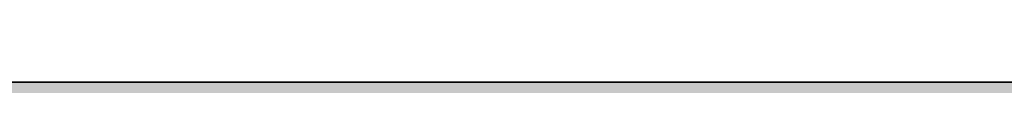
# Model space of a CAD drawing. Units: inches. Extents: x 2091 to 2899, y 967 to 2217.
# Tile 87 of 256: x 2251.287593 to 2251.296488, y 1099.919027 to 1099.919418. Entities that reach past the tile are written whole.
import ezdxf

# ---------------------------------------------------------------- set-up
doc = ezdxf.new("R2010")
doc.units = ezdxf.units.IN
doc.layers.add('A-WALL-PATT', color=141, linetype='Continuous', lineweight=13, true_color=0xadddf7)
doc.layers.add('L-SITE-WALL', color=7, linetype='Continuous', lineweight=35)

msp = doc.modelspace()

# ---------------------------------------------------------------- hatches: boundary and pattern name
at = {"layer": 'A-WALL-PATT'}
h = msp.add_hatch(color=256, dxfattribs=at)
h.dxf.hatch_style = 1
h.paths.add_polyline_path([(2212.1436027, 1941.4190588), (2387.6436027, 1941.4190588), (2387.6436027, 1824.4190588), (2392.1436027, 1824.4190588), (2392.1436027, 1941.4190588), (2609.6436027, 1941.4190588), (2609.6436027, 1825.9190588), (2614.1436027, 1825.9190588), (2614.1436027, 1941.4190588), (2794.1436027, 1941.4190588), (2794.1436027, 1928.7621663), (2803.1436027, 1928.7621663), (2803.1436027, 2050.9190588), (2203.1436027, 2050.9190588), (2203.1436027, 1900.7578592), (2212.1436027, 1900.7578592)])
h.paths.add_polyline_path([(2212.1436027, 1945.9190588), (2212.1436027, 2041.9190588), (2794.1436027, 2041.9190588), (2794.1436027, 1945.9190588), (2402.2482445, 1945.9190588), (2401.1024337, 1945.7758325), (2398.7024337, 1945.7758325)], flags=16)
h.paths.add_polyline_path([(2230.2298609, 1948.0627926), (2227.3498609, 1949.5027926), (2225.9098609, 1951.9027926), (2223.9898609, 1952.8627926), (2223.0298609, 1955.2627926), (2222.0698609, 1959.5827926), (2222.0698609, 1963.4227926), (2223.0298609, 1965.6627926), (2223.9898609, 1965.3427926), (2225.58591, 1963.860747), (2226.9115333, 1964.9572589), (2226.9488609, 1965.9387926), (2227.7783187, 1966.9521426), (2228.1999161, 1968.8787044), (2230.7098609, 1964.8627926), (2233.5898609, 1966.3027926), (2233.607309, 1966.3318728), (2233.7726595, 1964.9382048), (2234.6338015, 1963.6764729), (2235.0298609, 1963.9027926), (2236.2820348, 1965.5723578), (2235.9898609, 1962.9427926), (2237.9545121, 1957.5400019), (2238.3898609, 1957.9027926), (2239.2158609, 1960.3057926), (2238.6545655, 1966.3849599), (2238.6927918, 1966.4380694), (2238.8405779, 1967.4997069), (2238.7802908, 1967.6874864), (2238.8805378, 1967.7867629), (2238.6668609, 1966.2517926), (2239.2158609, 1960.3057926), (2238.3898609, 1957.9027926), (2236.9498609, 1956.7027926), (2234.5498609, 1949.9827926)], flags=0)
h.paths.add_polyline_path([(2278.0119735, 1948.0627926), (2276.4964266, 1947.8733492), (2275.8498328, 1947.6886081), (2274.6519735, 1947.1027926)], flags=0)
h.paths.add_polyline_path([(2269.8519735, 1955.7427926), (2268.2761762, 1956.6293287), (2270.8673022, 1956.3483982), (2269.3719735, 1958.1427926), (2268.7149641, 1959.1923253), (2270.5698328, 1958.7286081), (2268.5807252, 1961.9060872), (2270.8119735, 1960.8918835), (2270.8119735, 1963.4227926), (2271.3933148, 1964.7792556), (2270.2917623, 1966.1561963), (2271.7719735, 1965.6627926), (2272.1413868, 1966.5247568), (2273.9298328, 1965.9286081), (2275.6303855, 1968.054299), (2276.331938, 1966.72186), (2276.5204313, 1966.9521426), (2276.9420286, 1968.8787044), (2277.7342926, 1967.6110821), (2278.1398879, 1969.4645199), (2279.6591239, 1967.0337425), (2280.4119735, 1966.7827926), (2280.9493019, 1967.5887851), (2281.6098328, 1967.3686081), (2282.1332658, 1968.1537576), (2282.3492351, 1966.3334449), (2282.3498491, 1966.3325853), (2283.40755, 1968.0954201), (2283.7126314, 1965.5240203), (2284.3202211, 1964.6337894), (2284.5118085, 1964.8892393), (2284.2349735, 1965.7047926), (2284.500472, 1967.3189584), (2284.9079444, 1965.4174205), (2285.3963134, 1966.0685791), (2285.4328328, 1966.2906081), (2285.4733384, 1966.1712791), (2286.3539194, 1967.345387), (2286.2220067, 1966.1581734), (2287.6634921, 1968.0801538), (2287.7139735, 1968.4427926), (2288.4815994, 1969.0166793), (2288.5739928, 1968.7288966), (2288.9174612, 1969.0690403), (2288.6068328, 1966.8376081), (2288.9287261, 1963.3513103), (2288.9349735, 1963.3567926), (2288.9297314, 1963.3404224), (2289.015281, 1962.4138692), (2290.1112234, 1963.8751258), (2290.1328328, 1963.9426081), (2290.2176723, 1964.0170576), (2290.1112234, 1963.8751258), (2289.1558328, 1960.8916081), (2288.5940356, 1959.2572271), (2288.5719735, 1959.1027926), (2289.5319735, 1960.5427926), (2290.0119735, 1962.4627926), (2290.1918401, 1962.6426592), (2289.7698328, 1959.6886081), (2286.8898328, 1957.2886081), (2284.4898328, 1950.5686081), (2283.3146576, 1950.046308), (2283.2919735, 1949.9827926), (2280.2900585, 1948.6486081), (2281.1298328, 1948.6486081), (2282.5698328, 1948.1686081), (2283.2047262, 1948.0627926), (2278.9719735, 1948.0627926), (2276.0919735, 1949.5027926), (2274.6519735, 1951.9027926), (2272.7319735, 1952.8627926)], flags=0)
h.paths.add_polyline_path([(2271.1588684, 1958.0217654), (2272.9698328, 1955.8486081), (2272.0098328, 1960.1686081), (2272.0098328, 1964.0086081), (2272.6244258, 1965.4426583), (2274.3280226, 1963.860747), (2275.6536458, 1964.9572589), (2275.6377429, 1964.5390903), (2277.4122311, 1966.0068885), (2277.0329735, 1965.1567926), (2276.829924, 1964.9755966), (2276.7660116, 1963.2950136), (2277.4496351, 1962.6602203), (2279.4519735, 1964.8627926), (2282.3319735, 1966.3027926), (2283.5298328, 1966.8886081), (2283.2945117, 1966.7709476), (2283.9129934, 1963.8846999), (2284.8992493, 1964.4482747), (2284.7319735, 1962.9427926), (2286.6966247, 1957.5400019), (2287.1319735, 1957.9027926), (2287.5419128, 1959.0953883), (2287.7793955, 1958.4423109), (2285.6827383, 1956.6950966), (2285.8765033, 1959.7953357), (2284.7319735, 1962.9427926), (2284.8992493, 1964.4482747), (2283.9129934, 1963.8846999), (2284.2238328, 1962.4341157), (2283.4243649, 1963.6054836), (2281.6098328, 1962.5686081), (2281.1298328, 1960.1686081), (2282.0898328, 1956.3286081), (2283.0498328, 1952.9686081), (2282.5698328, 1950.5686081), (2280.1698328, 1948.6486081), (2279.883316, 1948.7918666), (2278.9719735, 1948.0627926), (2278.9719735, 1949.0227926), (2278.6723132, 1949.3973679), (2277.2898328, 1950.0886081), (2275.8498328, 1952.4886081), (2273.9298328, 1953.4486081), (2272.4898328, 1954.8886081), (2271.9216473, 1954.8886081), (2271.7719735, 1955.2627926)], flags=0)
h.paths.add_polyline_path([(2311.994146, 1955.7427926), (2312.0627174, 1955.6742211), (2312.0550999, 1955.7085002)], flags=0)
h.paths.add_polyline_path([(2331.956146, 1963.9517926), (2333.396146, 1965.3917926), (2331.077146, 1963.3567926), (2330.998603, 1963.1115166)], flags=0)
h.paths.add_polyline_path([(2310.554146, 1954.3027926), (2307.0398066, 1956.2799434), (2310.7629029, 1955.8762843), (2312.474146, 1953.8227926), (2313.434146, 1951.4227926), (2315.354146, 1950.4627926), (2316.794146, 1948.0627926), (2317.466146, 1947.7267926), (2319.3686915, 1947.9646108), (2317.754146, 1949.9827926), (2317.5695306, 1950.6104849), (2316.794146, 1951.9027926), (2314.874146, 1952.8627926), (2313.914146, 1955.2627926), (2311.514146, 1958.1427926), (2309.3754889, 1961.5591681), (2311.514146, 1960.3370783), (2311.514146, 1961.9827926), (2310.6046723, 1963.1196347), (2311.726605, 1962.4785303), (2312.4183321, 1964.09256), (2312.2559642, 1964.2955198), (2313.194146, 1963.9827926), (2313.914146, 1965.6627926), (2314.6467776, 1965.418582), (2315.354146, 1966.3027926), (2316.794146, 1967.7427926), (2316.1574354, 1966.9469043), (2317.0341105, 1965.28186), (2317.2226038, 1965.5121426), (2317.7770481, 1968.0457711), (2318.4741105, 1966.72186), (2318.6626038, 1966.9521426), (2319.0842012, 1968.8787044), (2321.2070492, 1965.4821474), (2322.1614187, 1966.9137017), (2322.554146, 1966.7827926), (2322.7859877, 1967.1305552), (2322.881646, 1966.3242926), (2323.3120408, 1965.7217399), (2323.6512889, 1965.891364), (2324.3964998, 1967.1333822), (2324.6569446, 1964.9382048), (2324.971986, 1964.476611), (2325.3872804, 1967.001499), (2325.9408127, 1964.4183481), (2327.2289286, 1966.1358361), (2327.1663199, 1965.5723578), (2328.0591386, 1966.7627827), (2328.2245759, 1966.2474864), (2329.6679714, 1967.6769101), (2329.6645759, 1967.6874864), (2329.7648229, 1967.7867629), (2329.551146, 1966.2517926), (2330.100146, 1960.3057926), (2329.3328143, 1958.0734703), (2329.3130649, 1957.935225), (2329.634146, 1958.2027926), (2330.234146, 1959.1027926), (2330.714146, 1961.0227926), (2331.034146, 1961.3427926), (2330.714146, 1959.1027926), (2329.634146, 1958.2027926), (2329.274146, 1957.6627926), (2327.7121121, 1956.3610977), (2325.434146, 1949.9827926), (2324.3337687, 1949.493736), (2323.994146, 1948.5427926), (2319.674146, 1946.6227926), (2316.794146, 1948.0627926), (2315.354146, 1950.4627926), (2313.434146, 1951.4227926)], flags=0)
h.paths.add_polyline_path([(2321.3356845, 1947.9520233), (2321.114146, 1948.0627926), (2321.114146, 1949.0227926), (2319.194146, 1951.4227926), (2316.794146, 1959.5827926), (2316.6632369, 1959.5827926), (2315.354146, 1958.1427926), (2314.394146, 1958.1427926), (2313.1483033, 1958.7090847), (2312.954146, 1959.5827926), (2312.954146, 1960.8918835), (2315.834146, 1959.5827926), (2316.6632369, 1959.5827926), (2317.3147094, 1960.2994123), (2315.0301951, 1962.420747), (2316.3558184, 1963.5172589), (2316.3723369, 1963.9516153), (2316.4701951, 1963.860747), (2317.7958184, 1964.9572589), (2317.7552187, 1963.8896871), (2319.175146, 1965.1567926), (2319.4984065, 1965.8813724), (2321.114146, 1965.3427926), (2323.2358851, 1962.3723578), (2325.6863494, 1963.7726231), (2325.5427886, 1962.4805756), (2325.1987827, 1963.4940135), (2324.4785097, 1963.0824289), (2324.9260053, 1960.9941157), (2324.0780866, 1962.2364729), (2322.4147912, 1961.2860184), (2322.074146, 1959.5827926), (2323.034146, 1955.7427926), (2323.994146, 1952.3827926), (2323.514146, 1949.9827926), (2322.1427174, 1948.8856497), (2322.074146, 1948.5427926)], flags=0)
h.paths.add_polyline_path([(2320.2074794, 1963.3374592), (2320.154146, 1963.4227926), (2320.394146, 1963.5427926)], flags=0)
h.paths.add_polyline_path([(2353.8505274, 1965.8105004), (2354.0305274, 1965.7505004), (2354.3305274, 1966.4505004), (2354.3305274, 1966.9305004)], flags=0)
h.paths.add_polyline_path([(2359.0205825, 1969.0264122), (2359.0983824, 1968.9019323), (2359.2335274, 1969.5195004), (2359.2335274, 1969.9995004)], flags=0)
h.paths.add_polyline_path([(2358.2566937, 1966.6816724), (2357.983601, 1966.3480346), (2358.211267, 1966.1461745), (2358.4104918, 1966.3895678)], flags=0)
h.paths.add_polyline_path([(2357.7684731, 1966.0587777), (2357.7321997, 1965.1049667), (2357.751047, 1965.1205565), (2357.7695274, 1965.6065004), (2357.7695274, 1966.057843)], flags=0)
h.paths.add_polyline_path([(2359.1115274, 1965.3045004), (2359.1115274, 1964.8245004), (2359.8445274, 1966.4675004), (2359.8445274, 1966.9475004)], flags=0)
h.paths.add_polyline_path([(2360.2236843, 1966.6214493), (2360.6985274, 1969.3625004), (2360.6985274, 1969.8425004), (2360.2105274, 1967.0255004), (2360.2105274, 1966.6425004)], flags=0)
h.paths.add_polyline_path([(2363.4505274, 1967.8905004), (2363.4505274, 1968.3705004), (2362.4905274, 1966.9305004), (2362.6560446, 1966.6987763)], flags=0)
h.paths.add_polyline_path([(2364.4755226, 1966.0788259), (2365.8505274, 1968.3705004), (2365.8505274, 1968.8505004), (2364.4279755, 1966.4795806)], flags=0)
h.paths.add_polyline_path([(2366.3135274, 1965.8525004), (2366.3667086, 1965.6958291), (2366.8025274, 1968.3455004), (2366.8025274, 1968.8255004)], flags=0)
h.paths.add_polyline_path([(2367.16531, 1965.8035439), (2367.2905274, 1966.9305004), (2367.2905274, 1967.4105004), (2367.1027013, 1965.7200656)], flags=0)
h.paths.add_polyline_path([(2370.0365274, 1959.9735004), (2371.0135274, 1963.0245004), (2371.0135274, 1963.5045004), (2370.0365274, 1960.4535004)], flags=0)
h.paths.add_polyline_path([(2371.6105274, 1960.2105004), (2372.5705274, 1961.6505004), (2372.5705274, 1962.1305004), (2371.8025274, 1960.9785004)], flags=0)
h.paths.add_polyline_path([(2350.8736661, 1956.0050856), (2351.9305274, 1955.8905004), (2354.4905274, 1953.3305004), (2353.8505274, 1954.9305004), (2351.4505274, 1957.8105004), (2347.9355274, 1963.4255004), (2347.9355274, 1963.9055004), (2351.4505274, 1958.2905004), (2353.7050728, 1955.5850458), (2352.8905274, 1959.2505004), (2352.8905274, 1959.7305004), (2352.8905274, 1961.9247861), (2356.7305274, 1959.7305004), (2358.454471, 1961.6268384), (2354.8105274, 1965.0105004), (2355.0308552, 1965.2859102), (2358.6910907, 1961.8871201), (2361.5305274, 1965.0105004), (2364.3764954, 1966.4334844), (2364.5243939, 1965.1869106), (2365.454468, 1963.8241807), (2365.8810728, 1964.0679549), (2365.3705274, 1966.4505004), (2365.3705274, 1966.9305004), (2366.8105274, 1960.2105004), (2366.8105274, 1959.7305004), (2366.3887092, 1952.9814095), (2367.7705274, 1956.8505004), (2368.641225, 1957.5760818), (2366.8105274, 1962.6105004), (2366.8105274, 1963.0905004), (2368.7751785, 1957.6877097), (2369.2105274, 1958.0505004), (2370.0015924, 1960.3518674), (2369.4752319, 1966.0526677), (2369.5134582, 1966.1057772), (2369.514173, 1966.1109121), (2369.4752319, 1966.5326677), (2369.5134582, 1966.5857772), (2369.614635, 1967.3125914), (2369.1825274, 1968.6585004), (2369.1825274, 1969.1385004), (2369.6009573, 1967.8351942), (2369.7012042, 1967.9344708), (2369.7179468, 1968.054743), (2370.1451758, 1968.3741448), (2369.7787075, 1968.0112238), (2369.7012042, 1967.4544708), (2370.4681613, 1968.2140038), (2369.674936, 1967.2657706), (2369.514173, 1966.1109121), (2370.0365274, 1960.4535004), (2370.0365274, 1959.9735004), (2369.441756, 1958.2431909), (2370.6505274, 1959.2505004), (2371.0458215, 1962.0175592), (2371.1305274, 1962.1305004), (2370.6505274, 1958.7705004), (2367.7705274, 1956.3705004), (2365.3705274, 1949.6505004), (2362.0790988, 1948.1876432), (2363.4505274, 1947.7305004), (2361.0505274, 1947.7305004), (2360.0905274, 1947.7305004), (2357.1038607, 1947.3571671), (2360.0905274, 1948.2105004), (2358.1705274, 1949.1705004), (2356.7305274, 1951.5705004), (2354.8105274, 1952.5305004), (2351.9305274, 1955.4105004)], flags=0)
h.paths.add_polyline_path([(2361.0505274, 1948.6905004), (2359.1305274, 1951.0905004), (2356.7305274, 1959.2505004), (2355.7705274, 1959.2505004), (2352.8905274, 1960.5595913), (2352.8905274, 1961.4447861), (2355.8905274, 1959.7305004), (2356.7305274, 1959.7305004), (2356.837194, 1959.3678337), (2361.5305274, 1964.5305004), (2363.2484221, 1965.3894478), (2364.92531, 1963.0418047), (2362.4905274, 1961.6505004), (2362.0638607, 1959.5171671), (2362.9705274, 1955.8905004), (2363.9305274, 1952.5305004), (2363.9305274, 1952.0505004), (2363.4505274, 1949.6505004), (2361.0505274, 1947.7305004)], flags=0)
h.paths.add_polyline_path([(2359.1305274, 1951.5705004), (2359.2905274, 1951.3705004), (2361.0505274, 1954.4505004), (2361.0505274, 1954.9305004)], flags=0)
h.paths.add_polyline_path([(2357.2195274, 1966.5455004), (2356.7925274, 1968.8145004), (2356.7925274, 1969.2945004), (2357.2195274, 1967.0255004)], flags=0)
h.paths.add_polyline_path([(2361.0505274, 1954.4505004), (2361.5305274, 1958.7705004), (2361.5305274, 1959.2505004), (2361.0505274, 1954.9305004)], flags=0)
h.paths.add_polyline_path([(2402.5482874, 1948.4860764), (2402.3024337, 1948.4158325), (2402.5904337, 1948.4158325)], flags=0)
h.paths.add_polyline_path([(2394.1424337, 1956.0958325), (2395.6850518, 1954.5532144), (2396.7204952, 1953.9706788), (2396.0624337, 1955.6158325), (2395.2413811, 1956.6010956), (2395.8789043, 1956.4417148), (2395.1024337, 1959.9358325), (2395.1024337, 1963.7758325), (2396.0624337, 1966.0158325), (2397.0224337, 1965.6958325), (2398.6184828, 1964.2137869), (2399.9441061, 1965.3102988), (2399.9814337, 1966.2918325), (2400.8108915, 1967.3051825), (2401.2324888, 1969.2317443), (2403.5379492, 1965.5430077), (2403.9419843, 1967.3893156), (2404.7024337, 1967.1358325), (2405.4603284, 1966.0747799), (2406.6224337, 1966.6558325), (2406.6398818, 1966.6849127), (2406.8052323, 1965.2912447), (2406.9256943, 1965.1147456), (2407.3424337, 1964.9758325), (2407.8743256, 1965.7736703), (2408.1691004, 1964.3980547), (2409.3146076, 1965.9253977), (2409.2174583, 1965.0510538), (2409.4452323, 1963.1312447), (2410.3063743, 1961.8695128), (2410.7024337, 1962.0958325), (2411.4422687, 1963.0822792), (2411.1654337, 1963.8978325), (2411.6164263, 1966.6397566), (2411.7253645, 1966.7911093), (2411.8731507, 1967.8527468), (2411.8128636, 1968.0405263), (2411.9131106, 1968.1398028), (2411.6994337, 1966.6048325), (2412.2484337, 1960.6588325), (2413.2254337, 1963.7098325), (2414.3779002, 1964.7211603), (2414.5131507, 1965.6927468), (2414.4528636, 1965.8805263), (2414.5531106, 1965.9798028), (2414.3779002, 1964.7211603), (2414.5198172, 1964.8456973), (2414.3653645, 1964.6311093), (2414.3394337, 1964.4448325), (2414.8884337, 1958.4988325), (2414.0624337, 1956.0958325), (2412.6224337, 1954.8958325), (2410.1713699, 1948.0328538), (2410.0167194, 1948.0844039), (2405.9024337, 1946.2558325), (2405.9024337, 1947.2158325), (2405.2042519, 1948.0885598), (2404.2224337, 1948.4158325), (2403.2624337, 1948.4158325), (2400.3824337, 1949.8558325), (2399.6624337, 1951.0558325), (2397.9824337, 1952.7358325), (2397.0224337, 1953.2158325), (2395.6850518, 1954.5532144), (2392.6567764, 1956.2569078)], flags=0)
h.paths.add_polyline_path([(2409.0856501, 1964.4074407), (2409.1303635, 1964.2757154), (2409.2624337, 1964.4958325)], flags=0)
h.paths.add_polyline_path([(2397.7424337, 1961.6158325), (2398.7024337, 1963.8558325), (2399.6624337, 1963.5358325), (2401.4265631, 1965.7409942), (2401.7914151, 1966.5588003), (2402.0714337, 1965.0708325), (2402.8355074, 1964.3933667), (2403.2623982, 1964.9148999), (2403.3381187, 1964.771086), (2402.6155159, 1963.9762229), (2402.4986125, 1960.9022379), (2403.5429971, 1959.9324522), (2404.4132029, 1960.8896786), (2404.7024337, 1962.3358325), (2407.9163468, 1964.1723542), (2409.5202115, 1961.9269436), (2410.9870849, 1957.8930418), (2411.4224337, 1958.2558325), (2412.0479637, 1960.075625), (2412.4103407, 1959.0790883), (2411.6756205, 1958.4668215), (2411.6624337, 1958.2558325), (2411.6260701, 1958.4255295), (2409.9824337, 1957.0558325), (2407.5824337, 1950.3358325), (2403.2624337, 1948.4158325), (2403.2624337, 1949.3758325), (2401.3424337, 1951.7758325), (2399.4165078, 1958.3239806), (2397.7424337, 1959.0849234), (2397.7424337, 1959.9701182), (2397.1024337, 1960.3358325), (2397.7424337, 1960.0449234)], flags=0)
h.paths.add_polyline_path([(2405.9024337, 1952.9758325), (2405.9504337, 1953.4078325), (2406.0167194, 1953.1758325)], flags=0)
h.paths.add_polyline_path([(2449.817778, 1967.1140143), (2449.7523235, 1967.1358325), (2449.7937028, 1967.0779014)], flags=0)
h.paths.add_polyline_path([(2451.6976961, 1966.6181202), (2451.7408949, 1966.6901182), (2451.6920515, 1966.6656965)], flags=0)
h.paths.add_polyline_path([(2454.3436278, 1965.7375716), (2455.7523235, 1967.6158325), (2455.9923235, 1968.0958325), (2454.3644974, 1965.9253977)], flags=0)
h.paths.add_polyline_path([(2457.5473235, 1968.8638325), (2457.7873235, 1969.3438325), (2457.0543235, 1968.7958325), (2457.0076216, 1968.4603446)], flags=0)
h.paths.add_polyline_path([(2456.9217835, 1967.8566619), (2456.8022381, 1968.2290163), (2456.7230003, 1967.6598028)], flags=0)
h.paths.add_polyline_path([(2457.3023235, 1967.3768325), (2457.5423235, 1967.8568325), (2456.8103235, 1966.8398325), (2456.7405164, 1966.7002183), (2456.7490213, 1966.6081053)], flags=0)
h.paths.add_polyline_path([(2458.2753235, 1963.7098325), (2458.1553426, 1963.3351533), (2460.3543235, 1965.2648325), (2460.5943235, 1965.7448325)], flags=0)
h.paths.add_polyline_path([(2458.3923235, 1962.8158325), (2458.3640882, 1962.6181854), (2459.5923235, 1964.2558325), (2459.8323235, 1964.7358325)], flags=0)
h.paths.add_polyline_path([(2459.3523235, 1962.8158325), (2459.2723235, 1962.4958325), (2460.0723235, 1963.2958325), (2460.3123235, 1963.7758325)], flags=0)
h.paths.add_polyline_path([(2458.6803235, 1960.6078325), (2458.6323235, 1960.4158325), (2459.5923235, 1961.8558325), (2459.8323235, 1962.3358325)], flags=0)
h.paths.add_polyline_path([(2437.8381696, 1956.2426502), (2439.1923235, 1956.0958325), (2441.3523235, 1953.9358325), (2440.8723235, 1955.1358325), (2438.4723235, 1958.0158325), (2438.0715634, 1958.6560225), (2438.7123235, 1958.4958325), (2440.6395962, 1956.1831052), (2439.9123235, 1959.4558325), (2439.9123235, 1963.2958325), (2441.3523235, 1966.6558325), (2441.5923235, 1967.1358325), (2441.1123235, 1966.0158325), (2442.0723235, 1965.6958325), (2443.9889932, 1968.0916696), (2444.2413235, 1966.7508325), (2444.9168011, 1966.1519203), (2445.6765737, 1967.0801359), (2446.2553235, 1969.7248325), (2446.4953235, 1970.2048325), (2446.2823786, 1969.2317443), (2447.362672, 1967.5032748), (2447.7203235, 1969.5678325), (2447.9603235, 1970.0478325), (2447.4854804, 1967.3067814), (2448.7923235, 1965.2158325), (2448.4723235, 1964.8638325), (2448.5523235, 1964.7358325), (2451.4520515, 1966.1856965), (2451.615122, 1964.8112447), (2452.3079173, 1963.7961718), (2453.2345053, 1964.3256507), (2454.0723235, 1960.4158325), (2453.6286871, 1953.3176507), (2454.7923235, 1956.5758325), (2455.0323235, 1957.0558325), (2455.7188351, 1957.6279255), (2453.8323235, 1962.8158325), (2453.940966, 1963.7936155), (2453.3353235, 1965.5778325), (2453.8243235, 1968.5508325), (2454.0643235, 1969.0308325), (2453.5753235, 1966.0578325), (2454.0403331, 1964.6879188), (2453.8323235, 1962.8158325), (2455.7188351, 1957.6279255), (2456.3672068, 1958.1682353), (2457.0583235, 1960.1788325), (2457.2983235, 1960.6588325), (2456.4723235, 1958.2558325), (2457.7177289, 1959.2936703), (2457.6723235, 1958.9758325), (2454.8899506, 1956.6571884), (2453.6141416, 1953.0849234), (2453.5923235, 1952.7358325), (2453.3523235, 1952.2558325), (2453.3595962, 1952.3721961), (2452.6323235, 1950.3358325), (2452.3923235, 1949.8558325), (2449.203752, 1948.4386896), (2450.7123235, 1947.9358325), (2448.0723235, 1947.9358325), (2447.1123235, 1947.9358325), (2444.5523235, 1947.6158325), (2447.1995962, 1948.3721961), (2445.1923235, 1949.3758325), (2443.7523235, 1951.7758325), (2441.8323235, 1952.7358325), (2438.9523235, 1955.6158325)], flags=0)
h.paths.add_polyline_path([(2443.9923235, 1959.9358325), (2444.0403235, 1959.7726325), (2444.1215542, 1959.8619863)], flags=0)
h.paths.add_polyline_path([(2442.9123235, 1959.9358325), (2443.0323235, 1959.9358325), (2442.4456568, 1960.2024992)], flags=0)
h.paths.add_polyline_path([(2444.9829435, 1965.0196767), (2445.2793235, 1965.2648325), (2445.5193235, 1965.7448325), (2444.9939958, 1965.3102988)], flags=0)
h.paths.add_polyline_path([(2446.1333235, 1965.0298325), (2446.3303662, 1965.4714986), (2444.9703235, 1964.2578325), (2444.7303235, 1963.7778325)], flags=0)
h.paths.add_polyline_path([(2442.7923235, 1959.4558325), (2443.7523235, 1959.4558325), (2446.1523235, 1951.2958325), (2446.4123235, 1951.7508325), (2446.3923235, 1951.7758325), (2448.0805993, 1954.7303152), (2448.5523235, 1958.9758325), (2441.8323235, 1965.2158325), (2442.1549464, 1965.6191112), (2448.7923235, 1959.4558325), (2448.3123235, 1955.1358325), (2448.0723235, 1954.6558325), (2446.4123235, 1951.7508325), (2448.3123235, 1949.3758325), (2448.3123235, 1948.4158325), (2450.5408949, 1950.1986896), (2450.9523235, 1952.2558325), (2449.9923235, 1955.6158325), (2449.0323235, 1959.4558325), (2449.5123235, 1961.8558325), (2449.7523235, 1962.3358325), (2449.6749041, 1961.9487357), (2452.9945053, 1963.8456507), (2453.0644143, 1963.5194086), (2452.8846108, 1963.7828538), (2449.6749041, 1961.9487357), (2449.2723235, 1959.9358325), (2450.2323235, 1956.0958325), (2451.1923235, 1952.7358325), (2450.7123235, 1950.3358325), (2450.4723235, 1949.8558325), (2448.0723235, 1947.9358325), (2448.0723235, 1948.5358325), (2445.4323235, 1949.8558325), (2443.9923235, 1952.2558325), (2442.0723235, 1953.2158325), (2441.1123235, 1955.6158325), (2440.1523235, 1959.9358325), (2440.1523235, 1960.6558325)], flags=0)
h.paths.add_polyline_path([(2456.6923235, 1966.9858325), (2457.6083235, 1968.0808325), (2457.8483235, 1968.5608325), (2456.9323235, 1967.4658325)], flags=0)
h.paths.add_polyline_path([(2489.8965704, 1966.5802407), (2489.9429477, 1966.1893466), (2490.7474884, 1967.5302478), (2491.3191223, 1968.9511605)], flags=0)
h.paths.add_polyline_path([(2473.5624709, 1956.4071313), (2477.139981, 1956.0192567), (2476.955333, 1956.2408343), (2475.1080486, 1957.2801078), (2476.3474884, 1956.9702478), (2475.1869011, 1958.8242158), (2476.9191223, 1958.3911605), (2475.4116422, 1960.7992688), (2477.7874884, 1959.7193388), (2477.7874884, 1962.2502478), (2477.637399, 1962.4378595), (2477.8225502, 1962.3320588), (2478.3591223, 1963.5840603), (2478.3591223, 1963.6711605), (2477.3243485, 1964.9646278), (2478.7148258, 1964.5011354), (2479.3191223, 1965.9111605), (2480.2791223, 1965.5911605), (2481.7839654, 1967.4722144), (2482.1164884, 1965.7052478), (2482.8805621, 1965.027782), (2483.209305, 1965.4294079), (2483.2201695, 1965.7150902), (2483.0759397, 1965.9890218), (2483.7117624, 1966.7658076), (2484.1304884, 1968.6792478), (2484.7021223, 1970.1001605), (2484.4891774, 1969.1270723), (2486.5029044, 1965.9051092), (2487.3874884, 1965.6102478), (2488.1534195, 1966.7591445), (2488.717017, 1965.9701079), (2489.2000857, 1966.2116422), (2489.3306713, 1965.1109919), (2490.3939049, 1963.6224649), (2490.6607651, 1963.7749564), (2490.4939052, 1964.553636), (2490.9230629, 1963.9248409), (2491.3191223, 1964.1511605), (2491.3333892, 1964.1701831), (2491.2104884, 1964.5322478), (2491.2817559, 1964.9655369), (2491.425789, 1964.2933827), (2494.0764757, 1967.8276317), (2494.4979183, 1966.5149416), (2494.5981652, 1966.6142182), (2494.6894884, 1967.2702478), (2495.106748, 1967.5821964), (2495.1298393, 1967.7480749), (2495.0695522, 1967.9358543), (2495.1697991, 1968.0351309), (2495.0317768, 1967.0436325), (2495.7538179, 1967.7586844), (2494.9820531, 1966.6864374), (2494.9561223, 1966.5001605), (2495.4790212, 1960.8368513), (2495.9104884, 1962.1842478), (2496.4821223, 1963.6051605), (2496.0726945, 1962.3265891), (2496.7689042, 1962.9375364), (2496.5991223, 1962.7111605), (2496.1191223, 1959.3511605), (2496.7328731, 1960.2717868), (2496.9874884, 1961.2902478), (2497.5591223, 1962.7111605), (2497.0791223, 1960.7911605), (2496.5074884, 1959.3702478), (2495.5474884, 1957.9302478), (2492.7588421, 1955.6063759), (2490.8391223, 1950.2311605), (2490.2674884, 1948.8102478), (2485.9474884, 1946.8902478), (2483.0674884, 1948.3302478), (2481.6274884, 1950.7302478), (2479.7074884, 1951.6902478), (2476.8274884, 1954.5702478)], flags=0)
h.paths.add_polyline_path([(2485.5769732, 1948.3133919), (2485.5591223, 1948.3111605), (2485.5787582, 1948.3111605)], flags=0)
h.paths.add_polyline_path([(2478.6450633, 1954.5511605), (2478.1090419, 1956.963257), (2479.3191223, 1955.5111605), (2480.2791223, 1953.1111605), (2482.1991223, 1952.1511605), (2483.6391223, 1949.7511605), (2486.5191223, 1948.3111605), (2486.5191223, 1949.2711605), (2484.7393067, 1951.49593), (2484.0274884, 1950.2502478), (2481.6274884, 1958.4102478), (2482.3751479, 1959.2326733), (2482.1991223, 1959.8311605), (2483.1975724, 1960.9294556), (2479.7074884, 1964.1702478), (2480.6033578, 1965.2900847), (2481.8751714, 1964.109115), (2482.666387, 1964.7635825), (2482.6153591, 1963.4217978), (2482.9891988, 1963.0746609), (2484.0084884, 1963.9842478), (2484.6836065, 1965.4975071), (2484.5801223, 1965.4051605), (2485.3572683, 1967.1471126), (2485.1206453, 1965.7811968), (2486.4274884, 1963.6902478), (2488.1453831, 1964.5491952), (2489.822271, 1962.2015522), (2490.7474884, 1962.7302478), (2491.9996623, 1964.3998131), (2492.0760458, 1965.0872647), (2492.2128915, 1964.6841187), (2492.4853744, 1965.0474291), (2492.2791223, 1963.1911605), (2494.2437735, 1957.7883698), (2494.5625035, 1958.0539782), (2494.9334884, 1959.1332478), (2495.5051223, 1960.5541605), (2494.6791223, 1958.1511605), (2494.1074884, 1956.7302478), (2494.5625035, 1958.0539782), (2493.4085439, 1957.0923452), (2491.7074884, 1961.7702478), (2491.9996623, 1964.3998131), (2490.7474884, 1962.7302478), (2487.7120303, 1960.9957003), (2487.4791223, 1959.8311605), (2488.4391223, 1955.9911605), (2489.3991223, 1952.6311605), (2488.9191223, 1950.2311605), (2488.5769183, 1949.9573973), (2488.3474884, 1948.8102478), (2487.6517154, 1948.2536295), (2487.4791223, 1948.3111605), (2486.5191223, 1948.3111605), (2483.6391223, 1949.7511605), (2482.1991223, 1952.1511605), (2480.2791223, 1953.1111605), (2478.8391223, 1954.5511605)], flags=0)
h.paths.add_polyline_path([(2526.648252, 1966.9875242), (2526.5173429, 1967.0311605), (2526.6001016, 1966.9152985)], flags=0)
h.paths.add_polyline_path([(2528.4706401, 1966.4466558), (2528.5744858, 1966.619732), (2528.4570709, 1966.5610245)], flags=0)
h.paths.add_polyline_path([(2534.1333429, 1967.4961605), (2534.1566852, 1967.5428451), (2534.0598415, 1967.4082958)], flags=0)
h.paths.add_polyline_path([(2536.1619229, 1964.0506005), (2535.1573429, 1962.7111605), (2535.1008723, 1962.3158664), (2536.1173429, 1963.6711605), (2536.4205319, 1964.2775386)], flags=0)
h.paths.add_polyline_path([(2535.1573429, 1959.8311605), (2536.1173429, 1961.2711605), (2536.5973429, 1962.2311605), (2535.2533429, 1960.2151605)], flags=0)
h.paths.add_polyline_path([(2513.2490352, 1956.284796), (2516.2211807, 1955.9625552), (2514.9973429, 1957.4311605), (2514.1958227, 1958.7115406), (2515.4773429, 1958.3911605), (2516.9318884, 1956.645706), (2516.4373429, 1958.8711605), (2516.4373429, 1962.7111605), (2516.8726918, 1963.7269745), (2515.3464338, 1965.6347969), (2517.3973429, 1964.9511605), (2517.8773429, 1966.0711605), (2518.3573429, 1967.0311605), (2517.8773429, 1965.9111605), (2518.8373429, 1965.5911605), (2520.4865896, 1967.6527188), (2520.7663429, 1966.1661605), (2521.5304166, 1965.4886947), (2521.7814433, 1965.7953745), (2521.8009106, 1966.307268), (2521.4778037, 1966.9209358), (2521.2463429, 1967.1261605), (2521.1777006, 1967.4909132), (2521.4778037, 1966.9209358), (2522.0104166, 1966.4486947), (2522.2573857, 1966.7504173), (2522.7803429, 1969.1401605), (2523.2603429, 1970.1001605), (2523.0473981, 1969.1270723), (2524.6731324, 1966.5258974), (2526.0373429, 1966.0711605), (2526.7952377, 1965.0101079), (2527.9770709, 1965.6010245), (2528.1401415, 1964.2265727), (2528.6645901, 1963.4581589), (2529.3886157, 1963.8718878), (2529.3296653, 1964.1469896), (2529.4812835, 1963.9248409), (2529.8773429, 1964.1511605), (2529.9840096, 1964.2933827), (2529.7890531, 1965.2031796), (2530.0623998, 1964.397903), (2532.802483, 1968.0513473), (2533.1477728, 1966.9758543), (2533.2480198, 1967.0751309), (2533.3393429, 1967.7311605), (2533.6728477, 1967.9804929), (2533.7280198, 1968.0351309), (2533.5143429, 1966.5001605), (2534.0247176, 1960.9724963), (2534.5603429, 1962.6451605), (2535.0403429, 1963.6051605), (2534.0633429, 1960.5541605), (2533.2373429, 1958.1511605), (2534.2881537, 1959.0268362), (2534.1973429, 1958.3911605), (2531.5125972, 1956.1538724), (2529.3973429, 1950.2311605), (2528.9173429, 1949.2711605), (2526.4487715, 1948.1740177), (2527.4773429, 1947.8311605), (2530.3573429, 1947.3511605), (2524.5973429, 1947.3511605), (2521.7173429, 1948.7911605), (2520.2773429, 1951.1911605), (2518.3573429, 1952.1511605), (2515.4773429, 1955.0311605)], flags=0)
h.paths.add_polyline_path([(2523.9347601, 1967.1903084), (2523.6195125, 1966.4836893), (2523.7704999, 1966.2421094)], flags=0)
h.paths.add_polyline_path([(2518.8373429, 1953.1111605), (2517.8773429, 1955.5111605), (2516.8849834, 1959.9767785), (2516.9173429, 1959.9620696), (2516.9173429, 1962.0254462), (2520.7573429, 1959.8311605), (2522.0249486, 1961.2255267), (2518.3573429, 1964.6311605), (2519.0025888, 1965.4377179), (2520.433392, 1964.109115), (2521.3011199, 1964.8268709), (2521.2451575, 1963.3553327), (2525.6383068, 1959.2759798), (2526.0373429, 1961.2711605), (2529.3973429, 1963.1911605), (2530.6495168, 1964.8607257), (2530.6647196, 1964.9975502), (2530.6919561, 1964.9173115), (2531.0877777, 1965.4450736), (2530.9459855, 1964.1689435), (2530.6919561, 1964.9173115), (2529.3973429, 1963.1911605), (2526.3625042, 1961.456967), (2526.0373429, 1959.8311605), (2526.9973429, 1955.9911605), (2527.9573429, 1952.6311605), (2527.4773429, 1950.2311605), (2527.1344858, 1949.9568748), (2526.9739283, 1949.1540874), (2526.6973429, 1949.0311605), (2524.5973429, 1947.3511605), (2524.5973429, 1948.3111605), (2524.2773429, 1948.7111605), (2522.1973429, 1949.7511605), (2520.7573429, 1952.1511605)], flags=0)
h.paths.add_polyline_path([(2520.2773429, 1958.8711605), (2520.8533429, 1959.5047605), (2523.1573429, 1951.6711605), (2524.6138947, 1954.220126), (2524.5973429, 1954.0711605), (2522.6773429, 1950.7111605)], flags=0)
h.paths.add_polyline_path([(2559.3709104, 1966.3111605), (2559.3984114, 1966.324911), (2559.4019428, 1966.3452961)], flags=0)
h.paths.add_polyline_path([(2549.7709104, 1957.1911605), (2552.6509104, 1954.3111605), (2552.1339874, 1955.6034682), (2550.6109104, 1957.4311605), (2547.0959104, 1963.0461605), (2545.7759104, 1965.2061605), (2549.2909104, 1959.5911605), (2551.6909104, 1956.7111605), (2550.7929329, 1960.7520594), (2550.7309104, 1960.7802514), (2550.7309104, 1964.8711605), (2551.6909104, 1967.1111605), (2552.6509104, 1966.7911605), (2554.2469595, 1965.309115), (2555.0342517, 1965.9603371), (2555.5816714, 1966.6446117), (2555.6099104, 1967.3871605), (2556.4393682, 1968.4005106), (2556.8609656, 1970.3270723), (2559.3709104, 1966.3111605), (2560.6909104, 1964.1511605), (2562.4088052, 1965.0101079), (2561.6509104, 1966.0711605), (2560.3309104, 1968.2311605), (2561.7584966, 1966.2325398), (2562.3472126, 1967.1156138), (2562.433709, 1966.3865727), (2563.127798, 1965.3696043), (2563.5709104, 1965.5911605), (2563.5883585, 1965.6202407), (2563.3625433, 1967.5235403), (2563.7224894, 1965.8437921), (2565.0600013, 1968.0729787), (2564.7328616, 1965.1287215), (2565.1175771, 1963.3333827), (2567.4446216, 1966.4361087), (2567.315615, 1967.8333279), (2567.3538413, 1967.8864374), (2567.5016274, 1968.9480749), (2567.4413403, 1969.1358543), (2567.5415873, 1969.2351309), (2567.3279104, 1967.7001605), (2567.8769104, 1961.7541605), (2568.7466892, 1964.4703273), (2568.635615, 1965.6733279), (2568.6738413, 1965.7264374), (2568.8216274, 1966.7880749), (2568.7613403, 1966.9758543), (2568.8615873, 1967.0751309), (2568.6479104, 1965.5401605), (2568.7261271, 1964.6930264), (2568.8539104, 1964.8051605), (2568.7466892, 1964.4703273), (2568.8172361, 1963.7062615), (2568.9709104, 1963.9111605), (2568.8660747, 1963.1773104), (2569.1969104, 1959.5941605), (2568.3709104, 1957.1911605), (2566.9309104, 1955.9911605), (2564.6202721, 1949.5213733), (2564.6509104, 1949.5111605), (2564.6166247, 1949.5111605), (2564.5309104, 1949.2711605), (2560.2109104, 1947.3511605), (2557.3309104, 1948.7911605), (2556.0451961, 1950.9340177), (2556.0109104, 1950.9511605), (2555.8566247, 1951.2083034), (2553.9709104, 1952.1511605), (2551.0909104, 1955.0311605), (2546.6501439, 1957.5295149)], flags=0)
h.paths.add_polyline_path([(2567.0257941, 1959.3302303), (2567.0350071, 1959.3048946), (2567.0509104, 1959.3511605)], flags=0)
h.paths.add_polyline_path([(2551.9682875, 1962.5183736), (2553.0109104, 1964.9511605), (2553.9709104, 1964.6311605), (2555.5669595, 1963.149115), (2556.8925828, 1964.2456268), (2556.9299104, 1965.2271605), (2557.1439841, 1965.4886947), (2556.420066, 1966.1305566), (2556.3914211, 1966.1049947), (2556.3799104, 1966.1661605), (2556.420066, 1966.1305566), (2556.9519104, 1966.6051605), (2557.0921386, 1966.9194783), (2557.5708749, 1966.010228), (2557.7593682, 1966.2405106), (2557.4179104, 1964.6801605), (2556.8925828, 1964.2456268), (2556.8070892, 1961.997566), (2560.6909104, 1958.3911605), (2560.6355258, 1957.892699), (2560.8109104, 1957.1911605), (2561.7709104, 1953.8311605), (2561.2909104, 1951.4311605), (2559.1104226, 1949.6867703), (2559.1564842, 1949.6291933), (2563.0265202, 1951.3492093), (2562.6109104, 1949.2711605), (2560.2109104, 1947.3511605), (2560.2109104, 1948.3111605), (2559.2509104, 1949.5111605), (2558.8909104, 1949.5111605), (2558.8909104, 1949.9611605), (2558.2909104, 1950.7111605), (2558.0537011, 1951.5176722), (2556.9709104, 1952.8711605), (2555.0678801, 1959.3414636), (2552.0509104, 1961.0654462), (2552.0509104, 1962.4711605)], flags=0)
h.paths.add_polyline_path([(2588.3300486, 1958.3911605), (2588.6102476, 1958.1109615), (2588.5533615, 1958.3669489)], flags=0)
h.paths.add_polyline_path([(2594.745454, 1950.4930862), (2593.9575317, 1953.1720221), (2593.1300486, 1954.5511605), (2591.2100486, 1955.5111605), (2590.2500486, 1957.9111605), (2588.3090328, 1960.2403795), (2586.1773061, 1961.2093462), (2587.8500486, 1960.7911605), (2587.2534157, 1961.7442456), (2588.4413145, 1961.0654462), (2588.4413145, 1962.6555276), (2588.4216793, 1962.6653452), (2588.4413145, 1962.7111605), (2586.9140379, 1964.6202563), (2588.8770864, 1963.7279616), (2589.2900486, 1964.6915402), (2589.2900486, 1966.0711605), (2590.2500486, 1968.3111605), (2591.2100486, 1967.9911605), (2592.8060977, 1966.509115), (2594.131721, 1967.6056268), (2594.1690486, 1968.5871605), (2594.9985064, 1969.6005106), (2595.4201038, 1971.5270723), (2597.9300486, 1967.5111605), (2600.8100486, 1968.9511605), (2600.8274967, 1968.9802407), (2600.9928472, 1967.5865727), (2601.8539892, 1966.3248409), (2602.1071433, 1966.4695004), (2602.2363539, 1967.255069), (2602.3567153, 1966.6933827), (2603.5022225, 1968.2207257), (2603.2100486, 1965.5911605), (2605.1746998, 1960.1883698), (2605.506891, 1960.4651958), (2605.026019, 1965.6733279), (2605.0642453, 1965.7264374), (2605.2120315, 1966.7880749), (2605.1517444, 1966.9758543), (2605.2519913, 1967.0751309), (2605.3433145, 1967.7311605), (2605.9529049, 1968.1868979), (2605.8747531, 1969.0333279), (2605.9129794, 1969.0864374), (2606.0607656, 1970.1480749), (2606.0004785, 1970.3358543), (2606.1007255, 1970.4351309), (2605.8870486, 1968.9001605), (2606.4360486, 1962.9541605), (2605.6100486, 1960.5511605), (2605.9970364, 1960.8736504), (2606.5643145, 1962.6451605), (2608.2414939, 1964.1169415), (2608.0100486, 1963.1911605), (2607.0500486, 1961.7511605), (2606.6314856, 1961.402358), (2606.2013145, 1958.3911605), (2603.3213145, 1955.9911605), (2600.9213145, 1949.2711605), (2596.6013145, 1947.3511605), (2593.7213145, 1948.7911605), (2592.8573145, 1950.2311605), (2592.6500486, 1950.2311605)], flags=0)
h.paths.add_polyline_path([(2596.6013145, 1947.3511605), (2596.6013145, 1948.3111605), (2594.6813145, 1950.7111605), (2596.1549537, 1953.2900292), (2595.5300486, 1954.0711605), (2593.1992262, 1961.9959568), (2592.6513399, 1962.5047084), (2591.780151, 1963.0025306), (2593.2829868, 1964.2456268), (2593.3203145, 1965.2271605), (2594.1497723, 1966.2405106), (2594.5713696, 1968.1670723), (2596.1826506, 1965.5890227), (2596.9512732, 1966.4345076), (2598.0413145, 1966.0711605), (2598.7992092, 1965.0101079), (2599.9613145, 1965.5911605), (2599.9787626, 1965.6202407), (2600.144113, 1964.2265727), (2601.0052551, 1962.9648409), (2601.4013145, 1963.1911605), (2602.6534884, 1964.8607257), (2602.3613145, 1962.2311605), (2603.7927479, 1958.2947186), (2601.9776436, 1953.2124265), (2601.9462078, 1952.7094535), (2599.4687551, 1951.6083634), (2599.0013145, 1949.2711605)], flags=0)
h.paths.add_polyline_path([(2597.5613145, 1958.8711605), (2597.6709663, 1959.4194194), (2597.5950535, 1958.7362045)], flags=0)
h.paths.add_polyline_path([(2623.6663046, 1961.2543751), (2625.5191629, 1960.7911605), (2624.9655444, 1961.6755326), (2627.1991629, 1960.6602514), (2627.1991629, 1961.1511605), (2626.9591629, 1962.2311605), (2626.9591629, 1963.4911605), (2625.5823208, 1965.2122132), (2626.9591629, 1964.4254462), (2626.9591629, 1965.8311605), (2626.8691629, 1965.8611605), (2627.9191629, 1968.3111605), (2628.8791629, 1967.9911605), (2630.475212, 1966.509115), (2631.8008353, 1967.6056268), (2631.8381629, 1968.5871605), (2632.6676207, 1969.6005106), (2633.089218, 1971.5270723), (2635.5991629, 1967.5111605), (2638.4791629, 1968.9511605), (2638.496611, 1968.9802407), (2638.6619615, 1967.5865727), (2639.1762733, 1966.8330111), (2639.7802155, 1967.8395816), (2640.0258296, 1966.6933827), (2641.1713368, 1968.2207257), (2640.8791629, 1965.5911605), (2641.114265, 1964.9446299), (2641.4113368, 1965.3407257), (2641.3080991, 1964.4115861), (2642.8438141, 1960.1883698), (2643.2791629, 1960.5511605), (2644.0847364, 1962.8947358), (2643.7838674, 1966.1533279), (2643.8068345, 1966.185237), (2643.6006764, 1968.418053), (2643.5228121, 1968.6605812), (2643.7298799, 1970.1480749), (2643.6695928, 1970.3358543), (2643.7698398, 1970.4351309), (2643.5561629, 1968.9001605), (2643.6006764, 1968.418053), (2643.9095928, 1967.4558543), (2644.0098398, 1967.5551309), (2643.8117426, 1966.1320789), (2644.1051629, 1962.9541605), (2644.2387733, 1961.3508359), (2644.7191629, 1961.7511605), (2645.0328526, 1962.2216951), (2645.3221629, 1963.1251605), (2646.0764203, 1963.7870466), (2645.0328526, 1962.2216951), (2644.3451629, 1960.0741605), (2643.5191629, 1957.6711605), (2642.0791629, 1956.4711605), (2639.7196124, 1949.864419), (2639.8755265, 1949.8384333), (2635.3591629, 1947.8311605), (2632.4791629, 1949.2711605), (2631.0391629, 1951.6711605), (2629.1191629, 1952.6311605), (2628.1591629, 1955.0311605), (2625.7591629, 1957.9111605)], flags=0)
h.paths.add_polyline_path([(2627.8163058, 1956.5740177), (2627.3737084, 1958.565706), (2626.3763058, 1959.7625891), (2627.1991629, 1959.3511605), (2627.3737084, 1958.565706), (2627.9191629, 1957.9111605), (2628.8791629, 1955.5111605), (2630.7991629, 1954.5511605), (2632.2391629, 1952.1511605), (2633.315025, 1951.6132295), (2631.0391629, 1959.3511605), (2631.4978296, 1959.8556939), (2630.7991629, 1962.2311605), (2631.4498671, 1962.9469352), (2630.715212, 1963.629115), (2632.0408353, 1964.7256268), (2632.0781629, 1965.7071605), (2632.2922366, 1965.9686947), (2631.7053393, 1966.4890671), (2633.136441, 1967.7661442), (2633.329218, 1968.6470723), (2634.6747185, 1966.4942716), (2635.2084652, 1967.0813931), (2636.7991629, 1966.5511605), (2637.6764043, 1967.8670226), (2638.9939455, 1966.0224649), (2639.7053447, 1966.4289787), (2641.1191629, 1959.8311605), (2640.930072, 1956.805706), (2639.4391629, 1952.6311605), (2638.2274556, 1952.0926239), (2637.7591629, 1949.7511605), (2635.3591629, 1947.8311605), (2635.3591629, 1948.7911605), (2633.4391629, 1951.1911605), (2633.315025, 1951.6132295), (2632.2391629, 1952.1511605), (2630.7991629, 1954.5511605), (2628.8791629, 1955.5111605)], flags=0)
h.paths.add_polyline_path([(2637.7591629, 1953.8311605), (2637.2791629, 1955.5111605), (2636.3191629, 1959.3511605), (2636.7991629, 1961.7511605), (2639.2339455, 1963.1424649), (2637.5570576, 1965.4901079), (2638.7388909, 1966.0810245), (2638.9019615, 1964.7065727), (2639.7631035, 1963.4448409), (2636.7991629, 1961.7511605), (2636.5324962, 1960.4178272), (2637.0391629, 1958.3911605), (2637.9991629, 1955.0311605)], flags=0)
h.paths.add_polyline_path([(2668.5674074, 1951.4311605), (2667.6074074, 1953.8311605), (2665.2074074, 1956.7111605), (2662.2939034, 1961.365307), (2665.4474074, 1959.5911605), (2666.6474074, 1958.3911605), (2666.6474074, 1959.9751605), (2666.0583165, 1960.6820696), (2666.6474074, 1960.3454462), (2666.6474074, 1961.9911605), (2666.7000904, 1962.1140874), (2666.4074074, 1963.4311605), (2666.4074074, 1967.2711605), (2667.3674074, 1969.5111605), (2668.3274074, 1969.1911605), (2669.9234565, 1967.709115), (2671.2490798, 1968.8056268), (2671.2864074, 1969.7871605), (2672.1158652, 1970.8005106), (2672.5374626, 1972.7270723), (2675.0474074, 1968.7111605), (2677.9274074, 1970.1511605), (2677.9448556, 1970.1802407), (2678.110206, 1968.7865727), (2678.9713481, 1967.5248409), (2679.3674074, 1967.7511605), (2680.6195814, 1969.4207257), (2680.3274074, 1966.7911605), (2682.2920586, 1961.3883698), (2682.7274074, 1961.7511605), (2683.358306, 1963.5865711), (2683.232112, 1964.9533279), (2683.2703383, 1965.0064374), (2683.3932153, 1965.8891377), (2683.3599691, 1966.2492145), (2683.3578373, 1966.2558543), (2683.3592288, 1966.2572323), (2682.992112, 1970.2333279), (2683.0303383, 1970.2864374), (2683.1781244, 1971.3480749), (2683.1178373, 1971.5358543), (2683.2180843, 1971.6351309), (2683.0044074, 1970.1001605), (2683.3592288, 1966.2572323), (2683.4580843, 1966.3551309), (2683.3932153, 1965.8891377), (2683.413908, 1965.6650231), (2684.4238098, 1966.8722747), (2683.5534074, 1964.1541605), (2683.358306, 1963.5865711), (2683.7934074, 1958.8741605), (2682.9674074, 1956.4711605), (2681.5274074, 1955.2711605), (2680.1092256, 1951.3002514), (2680.0849332, 1950.9115729), (2679.9768456, 1950.9295875), (2679.1274074, 1948.5511605), (2674.8074074, 1946.6311605), (2671.9274074, 1948.0711605), (2670.4874074, 1950.4711605)], flags=0)
h.paths.add_polyline_path([(2671.9356833, 1953.2270226), (2671.6874074, 1953.3511605), (2670.2474074, 1955.7511605), (2668.3274074, 1956.7111605), (2667.3567408, 1959.1378272), (2669.5274074, 1958.1511605), (2670.4874074, 1958.1511605), (2671.4794074, 1959.2423605), (2670.6844017, 1961.9453802), (2668.8895992, 1963.6119824), (2667.3074074, 1964.3311605), (2668.5674074, 1963.9111605), (2668.8309369, 1964.2405723), (2670.2474074, 1963.4311605), (2672.4221405, 1965.8233669), (2672.7774626, 1967.4470723), (2673.2340741, 1966.7164939), (2674.4119193, 1968.0121236), (2673.9805644, 1965.5221094), (2675.2874074, 1963.4311605), (2675.5540741, 1963.5644939), (2675.9324074, 1965.4561605), (2676.2474074, 1965.3511605), (2677.0053022, 1964.2901079), (2678.1674074, 1964.8711605), (2679.6074074, 1967.2711605), (2680.3274074, 1963.9111605), (2680.3065524, 1963.5774798), (2680.3472425, 1963.4576072), (2680.8595814, 1964.1407257), (2680.5674074, 1961.5111605), (2681.1036237, 1960.0365659), (2678.8874074, 1953.8311605), (2677.0924779, 1953.033414), (2677.6874074, 1950.9511605), (2677.2074074, 1948.5511605), (2674.8074074, 1946.6311605), (2674.8074074, 1947.5911605), (2672.8874074, 1949.9911605)], flags=0)
h.paths.add_polyline_path([(2673.9845503, 1951.9111605), (2674.5674074, 1952.9311605), (2674.5674074, 1951.9111605), (2676.9674074, 1953.8311605), (2677.4474074, 1956.2311605), (2676.4874074, 1959.5911605), (2676.2474074, 1960.5511605), (2679.7295893, 1962.5409787), (2680.0592668, 1961.0024837), (2679.2113481, 1962.2448409), (2676.2474074, 1960.5511605), (2676.4874074, 1959.5911605), (2677.4474074, 1956.2311605), (2676.9674074, 1953.8311605), (2674.5674074, 1951.9111605)], flags=0)
h.paths.add_polyline_path([(2707.4792832, 1952.8146508), (2706.5192832, 1955.2146508), (2705.5592832, 1959.5346508), (2705.5592832, 1963.3746508), (2706.5192832, 1965.6146508), (2707.4792832, 1965.2946508), (2709.0753323, 1963.8126052), (2710.4009555, 1964.9091171), (2710.4382832, 1965.8906508), (2711.267741, 1966.9040008), (2711.6893383, 1968.8305626), (2714.1992832, 1964.8146508), (2717.0792832, 1966.2546508), (2717.0967313, 1966.283731), (2717.2620817, 1964.890063), (2718.1232238, 1963.6283311), (2718.5192832, 1963.8546508), (2719.7714571, 1965.524216), (2719.4792832, 1962.8946508), (2721.4439344, 1957.4918601), (2721.8792832, 1957.8546508), (2722.7052832, 1960.2576508), (2722.1439877, 1966.3368181), (2722.182214, 1966.3899276), (2722.3300002, 1967.4515651), (2722.2697131, 1967.6393446), (2722.36996, 1967.7386211), (2722.1562832, 1966.2036508), (2722.7052832, 1960.2576508), (2721.8792832, 1957.8546508), (2720.4392832, 1956.6546508), (2718.0392832, 1949.9346508), (2713.7192832, 1948.0146508), (2710.8392832, 1949.4546508), (2709.3992832, 1951.8546508)], flags=0)
h.paths.add_polyline_path([(2749.3012306, 1952.8146508), (2748.3412306, 1955.2146508), (2747.3812306, 1959.5346508), (2747.3812306, 1963.3746508), (2748.3412306, 1965.6146508), (2749.3012306, 1965.2946508), (2750.8972797, 1963.8126052), (2752.222903, 1964.9091171), (2752.2602306, 1965.8906508), (2753.0896884, 1966.9040008), (2753.5112858, 1968.8305626), (2756.0212306, 1964.8146508), (2758.9012306, 1966.2546508), (2758.9186787, 1966.283731), (2759.0840292, 1964.890063), (2759.9451712, 1963.6283311), (2760.3412306, 1963.8546508), (2761.5934045, 1965.524216), (2761.3012306, 1962.8946508), (2763.2658818, 1957.4918601), (2763.7012306, 1957.8546508), (2764.5272306, 1960.2576508), (2763.9659351, 1966.3368181), (2764.0041614, 1966.3899276), (2764.1519476, 1967.4515651), (2764.0916605, 1967.6393446), (2764.1919075, 1967.7386211), (2763.9782306, 1966.2036508), (2764.5272306, 1960.2576508), (2763.7012306, 1957.8546508), (2762.2612306, 1956.6546508), (2759.8612306, 1949.9346508), (2755.5412306, 1948.0146508), (2752.6612306, 1949.4546508), (2751.2212306, 1951.8546508)], flags=0)
h.paths.add_polyline_path([(2212.1436027, 1819.9345143), (2203.1436027, 1819.9345143), (2203.1436027, 1739.9795464), (2212.1436027, 1739.9795464), (2212.1436027, 1780.9190588), (2392.1436027, 1780.9190588), (2392.1436027, 1783.9190588), (2212.1436027, 1783.9190588)])
h.paths.add_polyline_path([(2803.1436027, 1847.9388214), (2794.1436027, 1847.9388214), (2794.1436027, 1785.4190588), (2609.6436027, 1785.4190588), (2493.8756095, 1785.4190588), (2493.8756095, 1780.9190588), (2609.6436027, 1780.9190588), (2794.1436027, 1780.9190588), (2794.1436027, 1696.9190588), (2609.3756095, 1696.9190588), (2609.3756095, 1742.9190588), (2604.8756095, 1742.9190588), (2604.8756095, 1644.4190588), (2609.3756095, 1644.4190588), (2609.3756095, 1692.4190588), (2794.1436027, 1692.4190588), (2794.1436027, 1668.1647374), (2803.1436027, 1668.1647374)])
h.paths.add_polyline_path([(2392.1436027, 1740.4190588), (2387.6436027, 1740.4190588), (2387.6436027, 1629.4190588), (2212.1436027, 1629.4190588), (2212.1436027, 1659.1562015), (2203.1436027, 1659.1562015), (2203.1436027, 1494.089439), (2212.1436027, 1494.089439), (2212.1436027, 1627.9190588), (2392.1436027, 1627.9190588)])
h.paths.add_polyline_path([(2457.8756095, 1780.9190588), (2453.3756095, 1780.9190588), (2453.3756095, 1644.4190588), (2568.8756095, 1644.4190588), (2568.8756095, 1648.9190588), (2457.8756095, 1648.9190588)])
h.paths.add_polyline_path([(2545.1436027, 1591.9190588), (2540.6436027, 1591.9190588), (2540.6436027, 1567.9190588), (2468.6436027, 1567.9190588), (2468.6436027, 1627.9190588), (2509.1436027, 1627.9190588), (2509.1436027, 1632.4190588), (2464.1436027, 1632.4190588), (2464.1436027, 1563.4190588), (2545.1436027, 1563.4190588)])
h.paths.add_polyline_path([(2268.6436027, 1555.9190588), (2212.1436027, 1555.9190588), (2212.1436027, 1551.4190588), (2268.6436027, 1551.4190588)], flags=17)
h.paths.add_polyline_path([(2212.1436027, 1413.2660941), (2203.1436027, 1413.2660941), (2203.1436027, 1233.0704045), (2212.1436027, 1233.0704045)])
h.paths.add_polyline_path([(2267.6436027, 1351.9190588), (2212.1436027, 1351.9190588), (2212.1436027, 1347.4190588), (2267.6436027, 1347.4190588)], flags=17)
h.paths.add_polyline_path([(2456.6436027, 1489.4190588), (2452.1436027, 1489.4190588), (2452.1436027, 1351.9190588), (2312.6436027, 1351.9190588), (2312.6436027, 1347.4190588), (2456.6436027, 1347.4190588)])
h.paths.add_polyline_path([(2472.3701706, 1455.4190588), (2467.8701706, 1455.4190588), (2467.8701706, 1347.4190588), (2472.3701706, 1347.4190588)])
h.paths.add_polyline_path([(2794.1436027, 1351.9190588), (2543.3701706, 1351.9190588), (2543.3701706, 1347.4190588), (2794.1436027, 1347.4190588)], flags=17)
h.paths.add_polyline_path([(2312.6436027, 1347.4190588), (2308.1436027, 1347.4190588), (2308.1436027, 1302.1617866), (2308.3419658, 1302.1643273), (2308.1436027, 1298.1692489), (2308.1436027, 1275.4190588), (2212.1436027, 1275.4190588), (2212.1436027, 1270.9190588), (2312.6436027, 1270.9190588)], flags=17)
h.paths.add_polyline_path([(2212.1436027, 1152.2470596), (2203.1436027, 1152.2470596), (2203.1436027, 1090.9190588), (2803.1436027, 1090.9190588), (2803.1436027, 1392.7135549), (2794.1436027, 1392.7135549), (2794.1436027, 1143.4190588), (2548.0324471, 1143.4190588), (2548.0324471, 1138.9190588), (2794.1436027, 1138.9190588), (2794.1436027, 1099.9190588), (2212.1436027, 1099.9190588)])
h.paths.add_polyline_path([(2471.5324471, 1266.3285285, 0.031658), (2467.0324471, 1269.9457858), (2467.0324471, 1143.4190588), (2471.5324471, 1143.4190588), (2471.5324471, 1148.8190588)], flags=17)
h.paths.add_polyline_path([(2803.1436027, 1587.3413924), (2794.1436027, 1587.3413924), (2794.1436027, 1473.5368999), (2803.1436027, 1473.5368999)])
h.paths.add_polyline_path([(2794.1436027, 1536.4190588), (2651.1436027, 1536.4190588), (2651.1436027, 1531.9190588), (2794.1436027, 1531.9190588)])
h.paths.add_polyline_path([(2614.1436027, 1620.4190588), (2609.6436027, 1620.4190588), (2609.6436027, 1536.4190588), (2614.1436027, 1536.4190588)])
h.paths.add_polyline_path([(2271.0827276, 1964.3172377), (2776.852968, 1964.3172377), (2776.852968, 2037.1696226), (2271.0827276, 2037.1696226)], flags=8)
h.paths.add_polyline_path([(2380.6492852, 1536.8241435), (2461.0408087, 1536.8241435), (2461.0408087, 1554.6525871), (2380.6492852, 1554.6525871)], flags=9)
h.paths.add_polyline_path([(2203.6550381, 1608.8153118), (2316.1184385, 1608.8153118), (2316.1184385, 1621.9183562), (2203.6550381, 1621.9183562)], flags=24)
h.paths.add_polyline_path([(2212.6772554, 1313.5041021), (2282.5915203, 1313.5041021), (2282.5915203, 1322.7452389), (2212.6772554, 1322.7452389)], flags=24)
h.paths.add_polyline_path([(2457.111976, 1114.778574), (2558.4815807, 1114.778574), (2558.4815807, 1142.2196823), (2457.111976, 1142.2196823)], flags=25)
h.paths.add_polyline_path([(2473.4423372, 1273.0100672), (2604.6412257, 1273.0100672), (2604.6412257, 1318.3469349), (2473.4423372, 1318.3469349)], flags=25)
h.paths.add_polyline_path([(2638.8763024, 1626.9774316), (2684.2503675, 1627.9767377), (2684.0384825, 1637.5974944), (2638.6644174, 1636.5981884)], flags=9)
h.paths.add_polyline_path([(2537.5905538, 1453.7934466), (2628.3895472, 1453.7934466), (2628.3895472, 1475.3448114), (2537.5905538, 1475.3448114)], flags=9)
h.paths.add_polyline_path([(2504.1376376, 1714.6323972), (2554.6471875, 1714.6323972), (2554.6471875, 1730.2377115), (2504.1376376, 1730.2377115)], flags=25)
h.paths.add_polyline_path([(2487.5011806, 1575.6518716), (2535.0971214, 1575.6518716), (2535.0971214, 1598.3776456), (2487.5011806, 1598.3776456)], flags=25)
h.paths.add_polyline_path([(2709.0994004, 1735.7102784), (2740.0166009, 1735.7102784), (2740.0166009, 1749.9376406), (2709.0994004, 1749.9376406)], flags=25)
h.paths.add_polyline_path([(2442.4384239, 1792.1716575), (2564.7288353, 1792.1716575), (2564.7288353, 1842.0001626), (2442.4384239, 1842.0001626)], flags=9)
h.paths.add_polyline_path([(2655.8158012, 1809.6440763), (2789.5201425, 1806.6937963), (2790.0849768, 1832.2916379), (2656.3806355, 1835.2419179)], flags=25)
h.paths.add_polyline_path([(2234.8426972, 1797.7201432), (2368.5928512, 1794.7688523), (2369.1607182, 1820.504132), (2235.4105642, 1823.4554229)], flags=9)
h.paths.add_polyline_path([(2245.1384659, 1644.0063348), (2398.4277329, 1640.6238997), (2398.9948417, 1666.3248199), (2245.7055747, 1669.7072549)], flags=9)
h.paths.add_polyline_path([(2306.1428474, 1431.1685186), (2413.7683138, 1428.7936873), (2414.3331481, 1454.3915289), (2306.7076817, 1456.7663602)], flags=9)
h.paths.add_polyline_path([(2306.834582, 1458.2331447), (2393.3804836, 1456.3234487), (2393.9328082, 1481.3543583), (2307.3869066, 1483.2640542)], flags=9)

# ---------------------------------------------------------------- linework, layer by layer
at = {"layer": 'L-SITE-WALL'}
msp.add_line((2794.1436027, 1099.9190588), (2212.1436027, 1099.9190588), dxfattribs=at)

doc.saveas('drawing.dxf')
